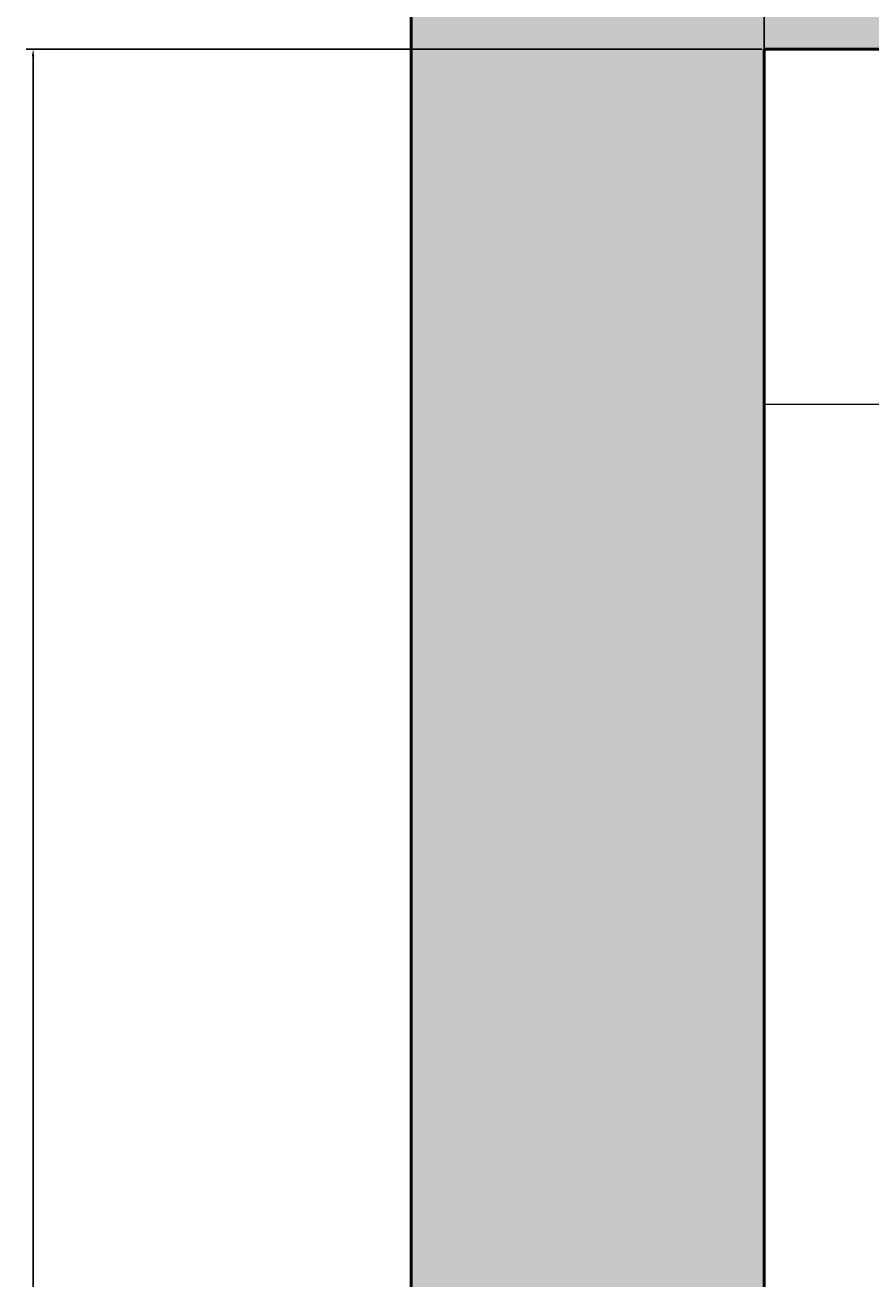
# Model space of a CAD drawing. Units: inches. Extents: x 2231 to 2461, y 2045 to 2455.
# Tile 49 of 95: x 2240 to 2262, y 2271 to 2303. Entities that reach past the tile are written whole.
import ezdxf

# ---------------------------------------------------------------- set-up
doc = ezdxf.new("R2010")
doc.units = ezdxf.units.IN
for name, color, linetype, lineweight in [('A-ANNO-DIMS', 2, 'Continuous', 18), ('A-FURN', 9, 'Continuous', 18), ('A-WALL', 7, 'Continuous', 50)]:
    doc.layers.add(name, color=color, linetype=linetype, lineweight=lineweight)
doc.layers.add('A-WALL-PATT', color=18, linetype='Continuous', lineweight=13, true_color=0x000000)
doc.styles.get("Standard").update_dxf_attribs({"font": 'arial.ttf'})
doc.dimstyles.get("Standard").update_dxf_attribs({"dimtxt": 0.18, "dimasz": 0.18, "dimexe": 0.18, "dimexo": 0.0625, "dimgap": 0.09, "dimtad": 0, "dimtih": 1, "dimtoh": 1, "dimdec": 4, "dimzin": 0, "dimdsep": 46, "dimtxsty": 'Standard', "dimcen": 0.09, "dimadec": 0, "dimazin": 0, "dimtfac": 1, "dimtdec": 4, "dimtofl": 0, "dimtmove": 0, "dimatfit": 3, "dimfxl": 1, "dimtolj": 1, "dimtzin": 0, "dimarcsym": 0})

# ---------------------------------------------------------------- blocks, each defined once
blk = doc.blocks.new('*D40')
at = {"layer": 'A-ANNO-DIMS', "color": 0, "lineweight": -2, "transparency": 16777216}
for p, q in [((2258.731, 2302.833), (2239.981, 2302.833)), ((2240.161, 2302.653), (2240.161, 2245.015)), ((2240.161, 2187.013), (2240.161, 2244.651)), ((2258.731, 2186.833), (2239.981, 2186.833))]:
    blk.add_line(p, q, dxfattribs=at)
at = {"layer": 'A-ANNO-DIMS', "color": 0, "transparency": 16777216}
for points in [[(2240.131, 2302.653), (2240.191, 2302.653), (2240.161, 2302.833)], [(2240.131, 2187.013), (2240.191, 2187.013), (2240.161, 2186.833)]]:
    blk.add_solid(points, dxfattribs=at)
at = {"layer": 'Defpoints', "color": 0, "transparency": 16777216}
for p in [(2240.161, 2302.833), (2258.794, 2302.833), (2258.794, 2186.833)]:
    blk.add_point(p, dxfattribs=at)
at = {"layer": 'A-ANNO-DIMS', "color": 0, "transparency": 16777216, "insert": (2240.161, 2244.833), "char_height": 0.18, "attachment_point": 5}
blk.add_mtext('\\A1;116', dxfattribs=at)
blk = doc.blocks.new('*D47')
at = {"layer": 'A-ANNO-DIMS', "color": 0, "lineweight": -2, "transparency": 16777216}
for p, q in [((2258.794, 2182.895), (2258.794, 2454.645)), ((2258.974, 2454.465), (2276.575, 2454.465)), ((2294.614, 2454.465), (2277.012, 2454.465)), ((2294.794, 2182.895), (2294.794, 2454.645))]:
    blk.add_line(p, q, dxfattribs=at)
at = {"layer": 'A-ANNO-DIMS', "color": 0, "transparency": 16777216}
for points in [[(2258.974, 2454.495), (2258.974, 2454.435), (2258.794, 2454.465)], [(2294.614, 2454.495), (2294.614, 2454.435), (2294.794, 2454.465)]]:
    blk.add_solid(points, dxfattribs=at)
at = {"layer": 'Defpoints', "color": 0, "transparency": 16777216}
for p in [(2294.794, 2454.465), (2258.794, 2182.833), (2294.794, 2182.833)]:
    blk.add_point(p, dxfattribs=at)
at = {"layer": 'A-ANNO-DIMS', "color": 0, "transparency": 16777216, "insert": (2276.794, 2454.465), "char_height": 0.18, "attachment_point": 5}
blk.add_mtext('\\A1;36', dxfattribs=at)
blk = doc.blocks.new('*D51')
at = {"layer": 'A-ANNO-DIMS', "color": 0, "lineweight": -2, "transparency": 16777216}
for p, q in [((2258.794, 2306.77), (2258.794, 2044.803)), ((2330.794, 2306.77), (2330.794, 2044.803)), ((2258.974, 2044.983), (2294.576, 2044.983)), ((2330.614, 2044.983), (2295.011, 2044.983))]:
    blk.add_line(p, q, dxfattribs=at)
at = {"layer": 'A-ANNO-DIMS', "color": 0, "transparency": 16777216}
for points in [[(2258.974, 2045.013), (2258.974, 2044.953), (2258.794, 2044.983)], [(2330.614, 2045.013), (2330.614, 2044.953), (2330.794, 2044.983)]]:
    blk.add_solid(points, dxfattribs=at)
at = {"layer": 'Defpoints', "color": 0, "transparency": 16777216}
for p in [(2258.794, 2306.833), (2330.794, 2306.833), (2330.794, 2044.983)]:
    blk.add_point(p, dxfattribs=at)
at = {"layer": 'A-ANNO-DIMS', "color": 0, "transparency": 16777216, "insert": (2294.794, 2044.983), "char_height": 0.18, "attachment_point": 5}
blk.add_mtext('\\A1;72', dxfattribs=at)

msp = doc.modelspace()

# ---------------------------------------------------------------- hatches: boundary and pattern name
at = {"layer": 'A-WALL-PATT'}
h = msp.add_hatch(color=256, dxfattribs=at)
h.dxf.hatch_style = 1
h.paths.add_polyline_path([(2441.7935, 2269.1535), (2432.7935, 2269.1535), (2432.7935, 2186.8328), (2396.7935, 2186.8328), (2396.7935, 2286.8328), (2394.7935, 2286.8328), (2394.7935, 2186.8328), (2334.7935, 2186.8328), (2334.7935, 2182.8328), (2432.7935, 2182.8328), (2432.7935, 2072.8328), (2416.6639, 2072.8328), (2416.6639, 2063.8328), (2441.7935, 2063.8328)])
h.paths.add_polyline_path([(2368.6639, 2072.8328), (2367.04, 2072.8328), (2330.7942, 2072.8328), (2330.7397, 2063.8328), (2368.6639, 2063.8328)])
h.paths.add_polyline_path([(2300.7392, 2068.3328), (2300.7392, 2072.8328), (2298.7935, 2072.8328), (2294.7935, 2072.8328), (2258.7935, 2072.8328), (2258.7935, 2120.8328), (2294.7935, 2120.8328), (2298.7935, 2120.8328), (2298.7935, 2128.8328), (2294.7935, 2128.8328), (2294.7935, 2124.8328), (2258.7935, 2124.8328), (2258.7935, 2182.8328), (2294.7935, 2182.8328), (2294.7935, 2174.8328), (2298.7935, 2174.8328), (2298.7935, 2182.8328), (2304.7935, 2182.8328), (2304.7935, 2186.8328), (2258.7935, 2186.8328), (2258.7935, 2221.999), (2249.7935, 2221.999), (2249.7935, 2063.8328), (2300.7392, 2063.8328)])
h.paths.add_polyline_path([(2391.9338, 2435.8328), (2333.82, 2435.8328), (2333.82, 2426.8328), (2368.7935, 2426.8328), (2368.7935, 2374.9508), (2368.7935, 2370.8328), (2372.3935, 2370.8328), (2372.7935, 2370.8328), (2372.7935, 2426.8328), (2391.9338, 2426.8328)])
h.paths.add_polyline_path([(2441.7935, 2435.8328), (2415.9338, 2435.8328), (2415.9338, 2426.8328), (2432.7935, 2426.8328), (2432.7935, 2334.8328), (2372.7935, 2334.8328), (2372.7935, 2346.8328), (2368.7935, 2346.8328), (2368.7935, 2306.8328), (2360.7935, 2306.8328), (2360.7935, 2302.8328), (2368.7935, 2302.8328), (2372.7935, 2302.8328), (2372.7935, 2330.8328), (2432.7935, 2330.8328), (2432.7935, 2317.1535), (2441.7935, 2317.1535)])
h.paths.add_polyline_path([(2285.82, 2435.8328), (2249.7935, 2435.8328), (2249.7935, 2269.999), (2258.7935, 2269.999), (2258.7935, 2302.8328), (2318.8168, 2302.8328), (2330.7935, 2302.8328), (2330.7935, 2306.8328), (2258.7935, 2306.8328), (2258.7935, 2426.8328), (2285.82, 2426.8328)])

# ---------------------------------------------------------------- linework, layer by layer
at = {"layer": 'A-FURN'}
msp.add_lwpolyline([(2258.7935, 2302.8328), (2318.8168, 2302.8328), (2318.8168, 2293.7759), (2258.7935, 2293.7759)], close=True, dxfattribs=at)
at = {"layer": 'A-WALL'}
for p, q in [((2258.7935, 2302.8328), (2330.7935, 2302.8328)), ((2258.7935, 2186.8328), (2258.7935, 2302.8328))]:
    msp.add_line(p, q, dxfattribs=at)
msp.add_lwpolyline([(2300.7392, 2063.8328), (2249.7935, 2063.8328), (2249.7935, 2435.8328), (2441.7935, 2435.8328), (2441.7935, 2063.8328), (2330.7397, 2063.8328)], dxfattribs=at)

# ---------------------------------------------------------------- dimensions: what is measured, and where the dimension line sits
at = {"layer": 'A-ANNO-DIMS'}
for base, p1, p2, picture, middle in [((2294.7935, 2454.4653), (2258.7935, 2182.8328), (2294.7935, 2182.8328), '*D47', (2276.7935, 2454.4653)), ((2330.7935, 2044.9825), (2258.7935, 2306.8328), (2330.7935, 2306.8328), '*D51', (2294.7935, 2044.9825))]:
    dim = msp.add_linear_dim(base=base, p1=p1, p2=p2, dimstyle='Standard', override={"dimdec": 0, "dimlfac": 1, "dimrnd": 0, "dimzin": 0, "dimdsep": 46, "dimlunit": 2}, dxfattribs=at)
    dim.commit()
    dim.dimension.update_dxf_attribs({"geometry": picture, "text_midpoint": middle})
dim = msp.add_linear_dim(base=(2240.161, 2302.8328), p1=(2258.7935, 2186.8328), p2=(2258.7935, 2302.8328), angle=90, dimstyle='Standard', override={"dimdec": 0, "dimlfac": 1, "dimrnd": 0, "dimzin": 0, "dimdsep": 46, "dimlunit": 2}, dxfattribs=at)
dim.commit()
dim.dimension.update_dxf_attribs({"geometry": '*D40', "text_midpoint": (2240.161, 2244.8328)})

doc.saveas('drawing.dxf')
